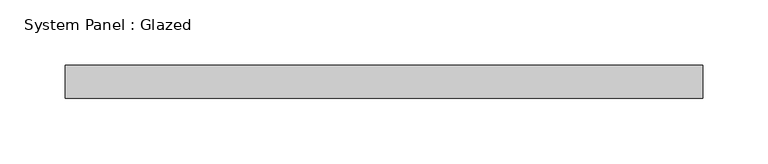
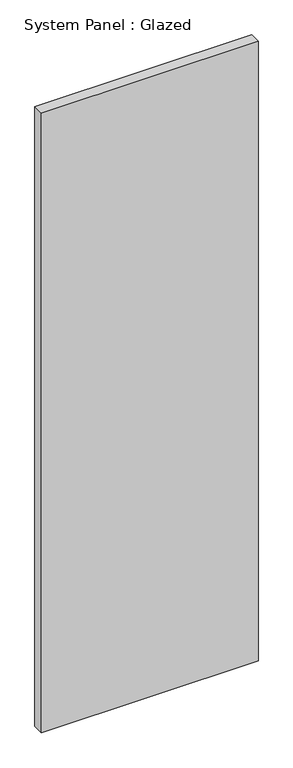
"""IFC4 building model written with IfcOpenShell, lengths in millimetres: plate geometry, System Panel : Glazed."""

from ifc_helpers import new_model, si_unit, origin, origin_with_axes, place, context, project, spatial, polyline, outline, extrude, source, transform, mapped, element, save


def system_panel_glazed_8ac636d5(model_context):
    return source(origin(), model_context, "Body", "SweptSolid", [
        extrude(outline(polyline([(244.475, 19.05), (-244.475, 19.05), (-244.475, 44.45), (244.475, 44.45), (244.475, 19.05)])), origin_with_axes(), (0.0, 0.0, 1.0), 1479.2683749),
    ])


if __name__ == "__main__":
    model = new_model("IFC4")
    model_context = context("Model", 3, world=origin())
    ifc_project = project(units=[si_unit("LENGTHUNIT", "METRE", prefix="MILLI")], contexts=[model_context])
    site = spatial("IfcSite", under=ifc_project)
    building = spatial("IfcBuilding", under=site)
    placement = place(None, origin())
    system_panel_glazed_shape = system_panel_glazed_8ac636d5(model_context)
    element("IfcPlate", 1, ObjectType="System Panel : Glazed", at=placement, inside=building, context=model_context, shape_type="MappedRepresentation", body=[
        mapped(system_panel_glazed_shape, transform((0.0, 0.0, 0.0), x_axis=(1.0, 0.0, 0.0), y_axis=(0.0, 1.0, 0.0), z_axis=(0.0, 0.0, 1.0))),
    ])
    save(model, "model.ifc")

# Revit data of these elements
# Type "System Panel : Glazed"
#   Construction Type Id = "GSP4R"
#   Analytic Construction = "1/8 in Pilkington single glazing"
#   Visual Light Transmittance = 0.9
#   Solar Heat Gain Coefficient = 0.86
#   Heat Transfer Coefficient (U) = 1.18115 BTU/(h·ft²·°F)
#   Define Thermal Properties by = 1
# Element 1 (IfcPlate, "System Panel : Glazed")
#   Materials on its faces: "Glass"
# Materials
#   "Glass": class "Glass", colour RGB 0 128 192, transparency 0.75, Description = "Soda Lime Glass", Cost = 0
